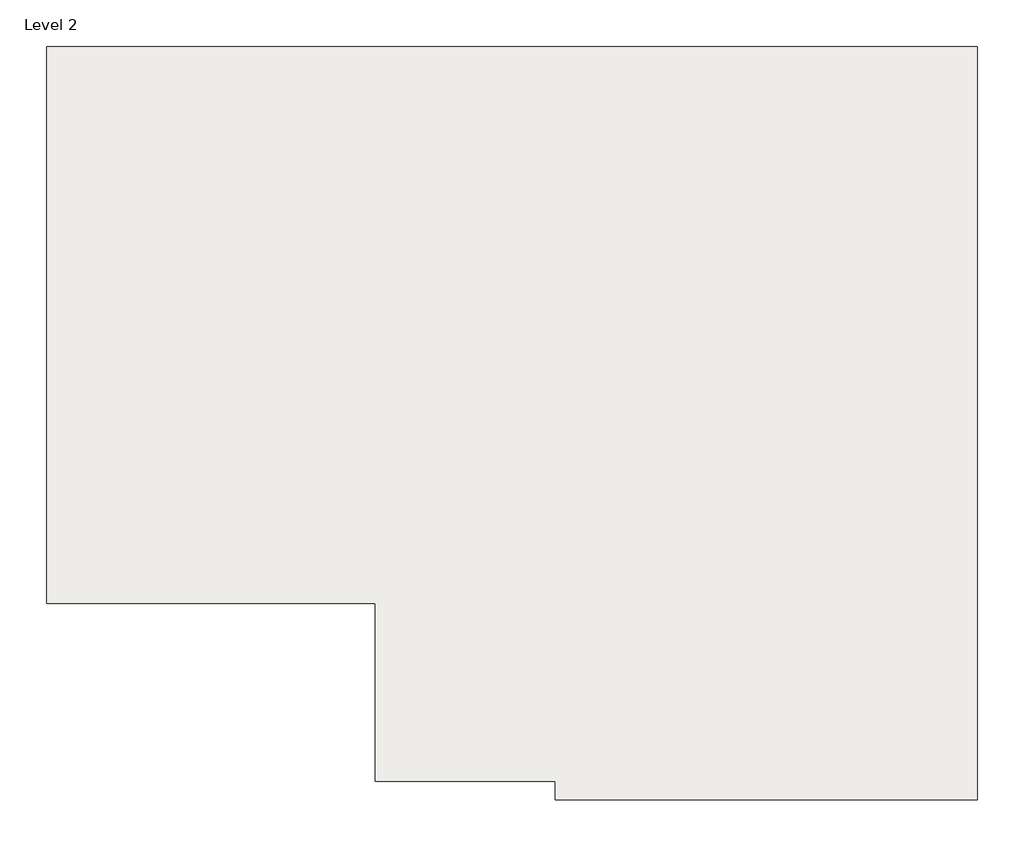
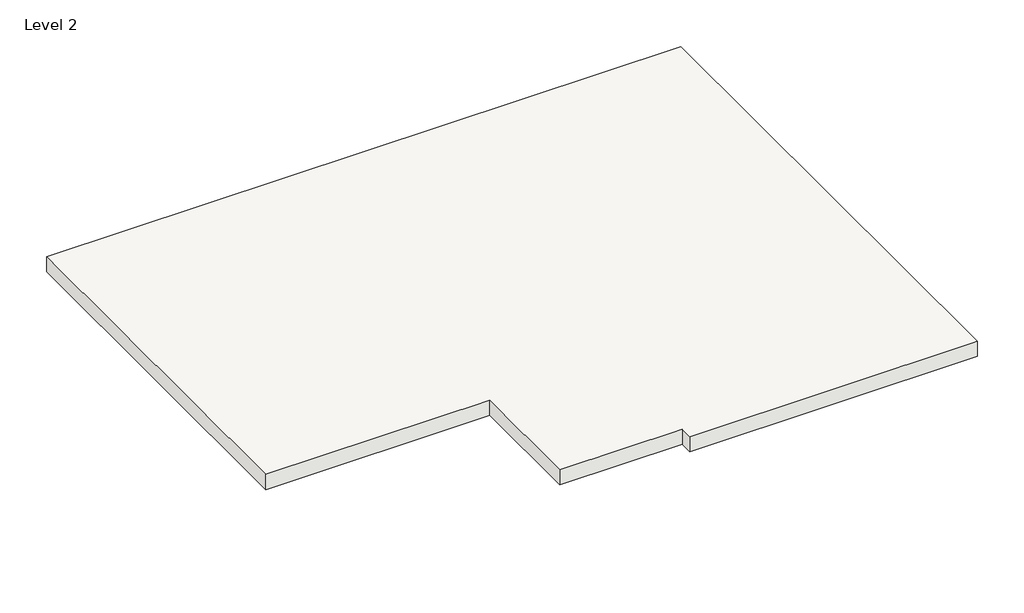
# One storey: 1 roof.
"""IFC4 building model written with IfcOpenShell, lengths in millimetres."""

from ifc_helpers import new_model, si_unit, frame, origin, place, context, project, spatial, polyline, outline, extrude, element, save

model = new_model("IFC4")

# Units and contexts
model_context = context("Model", 3, world=origin())
ifc_project = project(units=[si_unit("LENGTHUNIT", "METRE", prefix="MILLI")], contexts=[model_context])

# Site, building, storey
site = spatial("IfcSite", under=ifc_project)
building = spatial("IfcBuilding", under=site)
storey = spatial("IfcBuildingStorey", under=building, Name="Level 2", Elevation=3048.0)

# Roof
placement = place(None, origin())
element("IfcRoof", 1, ObjectType="Generic - 12\"", at=placement, inside=storey, context=model_context, shape_type="SweptSolid", body=[
    extrude(outline(polyline([(-14090.4576657, 13631.7729822), (-2000.0576657, 13631.7729822), (-2000.0576657, 3840.0729822), (-7486.4576657, 3840.0729822), (-7486.4576657, 4081.3729822), (-9823.2576657, 4081.3729822), (-9823.2576657, 6392.7729822), (-14090.4576657, 6392.7729822), (-14090.4576657, 13631.7729822)])), frame((0.0, 0.0, 3048.0), z_axis=(0.0, 0.0, 1.0), x_axis=(1.0, 0.0, 0.0)), (0.0, 0.0, 1.0), 304.8),
])

save(model, "model.ifc")

# Revit data of these elements
# Type "Generic - 12\""
#   Assembly Code = "B1020"
#   Layers, outside or top first: 1' - 0" "Brick, Soldier Course" (function 1)
# Element 1 (IfcRoof, "Generic - 12\"")
#   built-in parameter 1001705 = 11 (stored number, unit not read)
#   built-in parameter 1001710 = 33615
#   Phase Created = New Construction
#   Materials on its faces: "Brick, Soldier Course"
# Materials
#   "Brick, Soldier Course": class "Masonry", colour RGB 170 98 104, transparency 0, Description = "Common brick soldier coursed", Cost = 0
